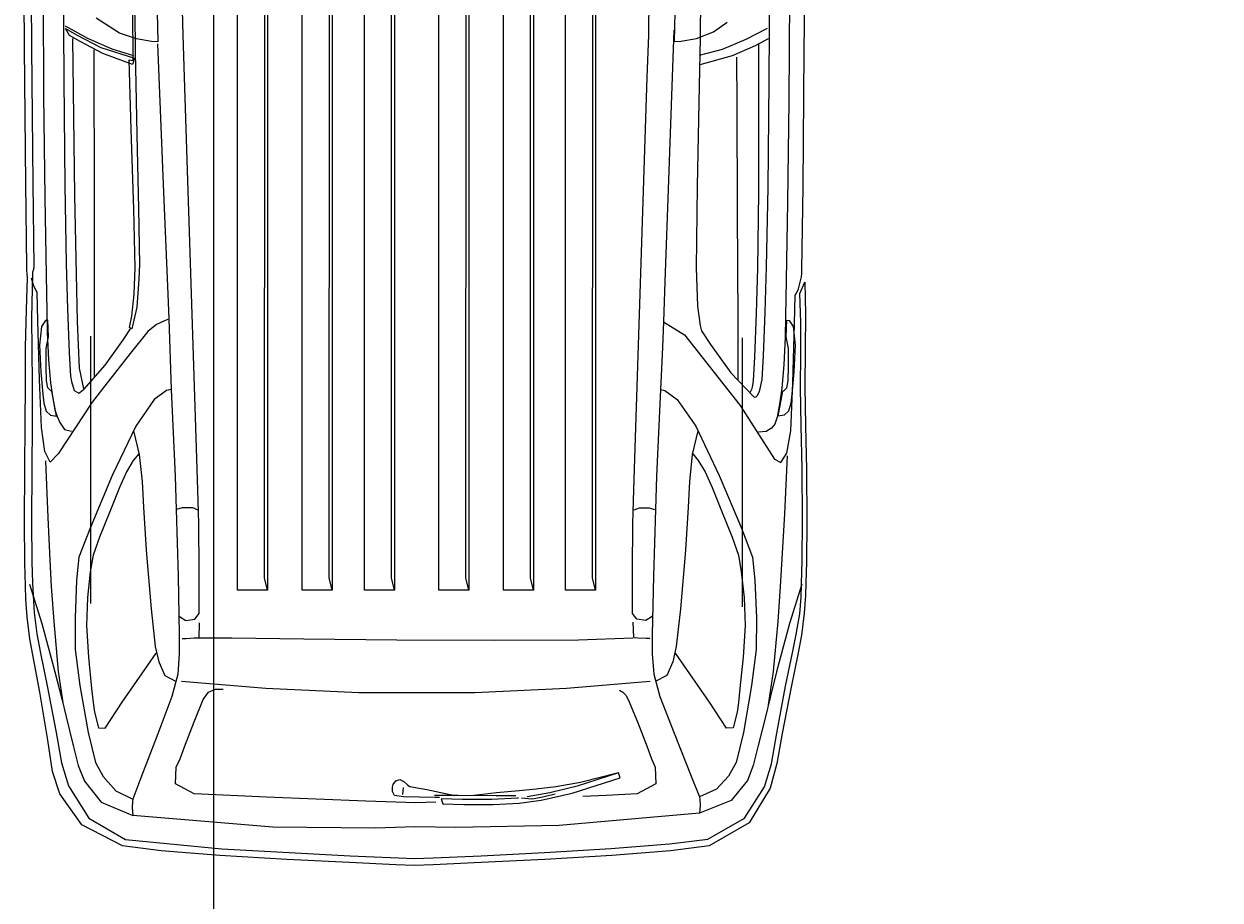
# Model space of a CAD drawing. Units: inches. Extents: x -4347 to -3836, y 955 to 1521.
# Tile 3 of 11: x -4130 to -4072, y 1023 to 1065. Entities that reach past the tile are written whole.
import ezdxf

# ---------------------------------------------------------------- set-up
doc = ezdxf.new("R2010")
doc.units = ezdxf.units.IN
doc.header["$MEASUREMENT"] = 0
doc.layers.add('A-ANNO-DIMS', color=2, linetype='Continuous', lineweight=18)
doc.layers.add('A-SITE-VEHC', color=8, linetype='Continuous', lineweight=13)
doc.styles.get("Standard").update_dxf_attribs({"font": 'arial.ttf'})
doc.dimstyles.get("Standard").update_dxf_attribs({"dimtxt": 0.18, "dimasz": 0.18, "dimexe": 0.18, "dimexo": 0.0625, "dimgap": 0.09, "dimtad": 0, "dimtih": 1, "dimtoh": 1, "dimdec": 0, "dimzin": 0, "dimdsep": 46, "dimlunit": 3, "dimtxsty": 'Standard', "dimcen": 0.09, "dimadec": 0, "dimazin": 0, "dimtfac": 1, "dimtdec": 0, "dimtofl": 0, "dimtmove": 0, "dimatfit": 3, "dimfxl": 1, "dimtolj": 1, "dimtzin": 0, "dimarcsym": 0})

# ---------------------------------------------------------------- blocks, each defined once
blk = doc.blocks.new('*D47')
at = {"layer": 'A-ANNO-DIMS', "color": 0, "lineweight": -2, "transparency": 16777216}
for p, q in [((-4120.58, 1288.726), (-4120.58, 966.959)), ((-3940.58, 1288.726), (-3940.58, 966.959)), ((-4120.4, 967.139), (-4030.97, 967.139)), ((-3940.76, 967.139), (-4030.189, 967.139))]:
    blk.add_line(p, q, dxfattribs=at)
at = {"layer": 'A-ANNO-DIMS', "color": 0, "transparency": 16777216}
for points in [[(-4120.4, 967.169), (-4120.4, 967.109), (-4120.58, 967.139)], [(-3940.76, 967.169), (-3940.76, 967.109), (-3940.58, 967.139)]]:
    blk.add_solid(points, dxfattribs=at)
at = {"layer": 'Defpoints', "color": 0, "transparency": 16777216}
for p in [(-4120.58, 1288.789), (-3940.58, 1288.789), (-3940.58, 967.139)]:
    blk.add_point(p, dxfattribs=at)
at = {"layer": 'A-ANNO-DIMS', "color": 0, "transparency": 16777216, "insert": (-4030.58, 967.139), "char_height": 0.18, "attachment_point": 5}
blk.add_mtext('\\A1;15\'-0"', dxfattribs=at)

msp = doc.modelspace()

# ---------------------------------------------------------------- linework, layer by layer
at = {"layer": 'A-SITE-VEHC'}
for p, q in [((-4119.421, 1037.674), (-4119.421, 1075.281)), ((-4117.988, 1075.281), (-4117.988, 1037.674)), ((-4117.987, 1075.281), (-4117.987, 1037.674)), ((-4116.333, 1037.674), (-4116.333, 1075.281)), ((-4114.9, 1075.281), (-4114.9, 1037.674)), ((-4114.899, 1075.281), (-4114.899, 1037.674)), ((-4113.355, 1037.674), (-4113.355, 1075.281)), ((-4111.923, 1075.281), (-4111.923, 1037.674)), ((-4111.921, 1075.281), (-4111.921, 1037.674)), ((-4109.792, 1037.674), (-4109.792, 1075.281)), ((-4108.36, 1075.281), (-4108.36, 1037.674)), ((-4108.359, 1075.281), (-4108.359, 1037.674)), ((-4106.704, 1037.674), (-4106.704, 1075.281)), ((-4105.272, 1075.281), (-4105.272, 1037.674)), ((-4105.271, 1075.281), (-4105.271, 1037.674)), ((-4103.727, 1037.674), (-4103.727, 1075.281)), ((-4102.293, 1075.281), (-4102.293, 1037.674)), ((-4118.131, 1038.272), (-4118.117, 1075.163)), ((-4115.043, 1038.272), (-4115.029, 1075.163)), ((-4112.065, 1038.272), (-4112.051, 1075.163)), ((-4108.503, 1038.272), (-4108.489, 1075.163)), ((-4105.415, 1038.272), (-4105.401, 1075.163)), ((-4102.436, 1038.272), (-4102.422, 1075.163)), ((-4127.755, 1067.874), (-4127.742, 1064.565)), ((-4123.32, 1068.019), (-4123.237, 1063.886)), ((-4098.438, 1067.866), (-4098.543, 1063.914)), ((-4097.264, 1067.866), (-4097.297, 1064.092)), ((-4094, 1067.678), (-4093.989, 1064.522)), ((-4129.614, 1063.599), (-4129.643, 1066.995)), ((-4129.312, 1066.995), (-4129.283, 1063.603)), ((-4092.31, 1063.442), (-4092.281, 1066.834)), ((-4128.73, 1066.524), (-4128.703, 1061.321)), ((-4093.024, 1066.275), (-4093.052, 1061.072)), ((-4124.346, 1065.547), (-4124.329, 1063.972)), ((-4122.033, 1064.207), (-4122.068, 1066.049)), ((-4099.752, 1064.207), (-4099.725, 1066.049)), ((-4125.067, 1064.303), (-4126.18, 1065.018)), ((-4124.412, 1063.007), (-4124.426, 1065.411)), ((-4127.742, 1064.565), (-4127.728, 1062.059)), ((-4127.664, 1064.666), (-4126.594, 1064.066)), ((-4127.466, 1064.193), (-4127.659, 1064.524)), ((-4127.659, 1064.524), (-4127.134, 1064.22)), ((-4098.545, 1064.449), (-4098.811, 1057.276)), ((-4097.463, 1064.047), (-4096.656, 1064.377)), ((-4096.656, 1064.377), (-4096.001, 1064.832)), ((-4094.088, 1064.533), (-4095.111, 1064.01)), ((-4093.989, 1064.522), (-4094.01, 1061.988)), ((-4126.958, 1063.902), (-4127.466, 1064.193)), ((-4127.314, 1064.055), (-4127.287, 1061.554)), ((-4127.134, 1064.22), (-4125.971, 1063.627)), ((-4125.876, 1063.33), (-4126.958, 1063.902)), ((-4126.594, 1064.066), (-4125.437, 1063.557)), ((-4124.25, 1064.035), (-4125.067, 1064.303)), ((-4124.329, 1063.972), (-4124.326, 1063.811)), ((-4124.326, 1063.811), (-4124.317, 1063.36)), ((-4123.54, 1063.914), (-4124.25, 1064.035)), ((-4123.237, 1063.886), (-4123.54, 1063.914)), ((-4123.249, 1063.791), (-4122.968, 1056.683)), ((-4121.96, 1062.197), (-4122.033, 1064.207)), ((-4099.825, 1062.197), (-4099.752, 1064.207)), ((-4098.543, 1063.914), (-4098.213, 1063.929)), ((-4098.213, 1063.929), (-4097.463, 1064.047)), ((-4097.297, 1064.092), (-4097.344, 1061.771)), ((-4095.111, 1064.01), (-4096.246, 1063.527)), ((-4094.642, 1063.721), (-4094.025, 1064.058)), ((-4129.553, 1057.123), (-4129.614, 1063.599)), ((-4129.283, 1063.603), (-4129.223, 1057.133)), ((-4126.294, 1063.504), (-4126.284, 1056.049)), ((-4125.971, 1063.627), (-4124.357, 1063.11)), ((-4124.453, 1062.815), (-4125.876, 1063.33)), ((-4125.437, 1063.557), (-4124.405, 1063.242)), ((-4124.317, 1063.36), (-4124.304, 1062.665)), ((-4096.246, 1063.527), (-4097.333, 1063.238)), ((-4097.297, 1062.811), (-4095.74, 1063.246)), ((-4095.74, 1063.246), (-4094.642, 1063.721)), ((-4094.504, 1063.766), (-4094.499, 1061.413)), ((-4092.371, 1056.974), (-4092.31, 1063.442)), ((-4124.508, 1059.696), (-4124.612, 1063.035)), ((-4124.612, 1063.035), (-4124.412, 1063.007)), ((-4124.357, 1063.11), (-4124.453, 1062.815)), ((-4124.304, 1062.665), (-4124.234, 1059.464)), ((-4095.552, 1063.159), (-4095.541, 1060.882)), ((-4121.831, 1058.246), (-4121.96, 1062.197)), ((-4099.954, 1058.246), (-4099.825, 1062.197)), ((-4127.728, 1062.059), (-4127.688, 1057.047)), ((-4127.287, 1061.554), (-4127.223, 1056.55)), ((-4097.344, 1061.771), (-4097.431, 1057.007)), ((-4094.01, 1061.988), (-4094.063, 1056.923)), ((-4128.703, 1061.321), (-4128.641, 1056.456)), ((-4094.499, 1061.413), (-4094.503, 1056.686)), ((-4093.052, 1061.072), (-4093.113, 1056.207)), ((-4095.541, 1060.882), (-4095.518, 1055.8)), ((-4124.39, 1055.896), (-4124.508, 1059.696)), ((-4124.234, 1059.464), (-4124.154, 1055.914)), ((-4121.675, 1053.327), (-4121.831, 1058.246)), ((-4100.11, 1053.327), (-4099.954, 1058.246)), ((-4129.501, 1053.135), (-4129.553, 1057.123)), ((-4129.223, 1057.133), (-4129.17, 1053.148)), ((-4127.688, 1057.047), (-4127.627, 1053.284)), ((-4098.811, 1057.276), (-4098.98, 1052.427)), ((-4097.431, 1057.007), (-4097.477, 1053.096)), ((-4094.063, 1056.923), (-4094.132, 1053.131)), ((-4092.423, 1052.989), (-4092.371, 1056.974)), ((-4128.641, 1056.456), (-4128.58, 1052.745)), ((-4127.223, 1056.55), (-4127.149, 1052.792)), ((-4122.968, 1056.683), (-4122.782, 1052.206)), ((-4094.503, 1056.686), (-4094.545, 1053.076)), ((-4126.284, 1056.049), (-4126.278, 1050.721)), ((-4124.323, 1053.082), (-4124.39, 1055.896)), ((-4124.154, 1055.914), (-4124.116, 1053.241)), ((-4095.518, 1055.8), (-4095.495, 1050.539)), ((-4093.113, 1056.207), (-4093.174, 1052.496)), ((-4129.496, 1052.966), (-4129.501, 1053.135)), ((-4129.488, 1052.798), (-4129.496, 1052.966)), ((-4129.19, 1053.009), (-4129.227, 1052.888)), ((-4129.17, 1053.148), (-4129.19, 1053.009)), ((-4127.627, 1053.284), (-4127.556, 1051.123)), ((-4124.365, 1051.837), (-4124.323, 1053.082)), ((-4124.116, 1053.241), (-4124.141, 1052.564)), ((-4121.518, 1048.41), (-4121.675, 1053.327)), ((-4100.267, 1048.41), (-4100.11, 1053.327)), ((-4097.477, 1053.096), (-4097.413, 1051.251)), ((-4094.545, 1053.076), (-4094.617, 1050.916)), ((-4094.132, 1053.131), (-4094.203, 1050.971)), ((-4092.434, 1052.819), (-4092.423, 1052.989)), ((-4129.527, 1051.074), (-4129.467, 1052.631)), ((-4129.467, 1052.631), (-4129.488, 1052.798)), ((-4129.165, 1052.211), (-4129.274, 1052.598)), ((-4129.231, 1052.751), (-4129.244, 1052.103)), ((-4129.227, 1052.888), (-4129.231, 1052.751)), ((-4128.58, 1052.745), (-4128.552, 1051.006)), ((-4127.149, 1052.792), (-4127.095, 1050.522)), ((-4124.141, 1052.564), (-4124.247, 1051.205)), ((-4098.98, 1052.427), (-4099.043, 1050.506)), ((-4093.174, 1052.496), (-4093.202, 1050.757)), ((-4092.581, 1052.09), (-4092.47, 1052.523)), ((-4092.519, 1051.868), (-4092.292, 1052.4)), ((-4092.47, 1052.523), (-4092.449, 1052.664)), ((-4092.449, 1052.664), (-4092.434, 1052.819)), ((-4092.292, 1052.4), (-4092.259, 1050.877)), ((-4129.244, 1052.103), (-4129.276, 1050.685)), ((-4129.061, 1051.997), (-4129.165, 1052.211)), ((-4129.015, 1051.931), (-4129.061, 1051.997)), ((-4128.983, 1050.56), (-4129.015, 1051.931)), ((-4124.477, 1050.777), (-4124.365, 1051.837)), ((-4122.782, 1052.206), (-4122.715, 1050.65)), ((-4092.775, 1050.408), (-4092.744, 1051.779)), ((-4092.744, 1051.779), (-4092.693, 1051.852)), ((-4092.693, 1051.852), (-4092.581, 1052.09)), ((-4092.48, 1050.469), (-4092.519, 1051.868)), ((-4124.247, 1051.205), (-4124.488, 1050.173)), ((-4097.413, 1051.251), (-4097.293, 1050.325)), ((-4129.562, 1049.313), (-4129.527, 1051.074)), ((-4129.276, 1050.685), (-4129.259, 1049.178)), ((-4128.552, 1051.006), (-4128.53, 1050.017)), ((-4127.556, 1051.123), (-4127.485, 1049.026)), ((-4126.278, 1050.721), (-4126.275, 1047.874)), ((-4124.598, 1050.228), (-4124.477, 1050.777)), ((-4122.759, 1050.623), (-4122.926, 1050.562)), ((-4122.715, 1050.65), (-4122.606, 1047.271)), ((-4094.617, 1050.916), (-4094.688, 1048.818)), ((-4094.203, 1050.971), (-4094.274, 1048.873)), ((-4093.202, 1050.757), (-4093.224, 1049.768)), ((-4092.259, 1050.877), (-4092.271, 1049.178)), ((-4128.904, 1047.75), (-4128.983, 1050.56)), ((-4128.805, 1050.286), (-4128.894, 1049.393)), ((-4128.605, 1050.569), (-4128.805, 1050.286)), ((-4128.493, 1050.586), (-4128.605, 1050.569)), ((-4128.473, 1049.788), (-4128.493, 1050.586)), ((-4127.095, 1050.522), (-4127.008, 1048.29)), ((-4124.53, 1050.223), (-4124.898, 1049.654)), ((-4124.488, 1050.173), (-4124.598, 1050.228)), ((-4123.712, 1050.045), (-4124.562, 1048.994)), ((-4123.304, 1050.372), (-4123.712, 1050.045)), ((-4122.926, 1050.562), (-4123.304, 1050.372)), ((-4099.043, 1050.506), (-4099.097, 1049.302)), ((-4099.043, 1050.506), (-4098.047, 1049.892)), ((-4097.293, 1050.325), (-4097.228, 1050.07)), ((-4097.228, 1050.07), (-4096.804, 1049.417)), ((-4095.495, 1050.539), (-4095.484, 1047.721)), ((-4093.173, 1049.788), (-4093.153, 1050.586)), ((-4093.153, 1050.586), (-4093.042, 1050.569)), ((-4093.042, 1050.569), (-4092.841, 1050.286)), ((-4092.854, 1047.597), (-4092.775, 1050.408)), ((-4092.841, 1050.286), (-4092.752, 1049.393)), ((-4092.483, 1048.998), (-4092.48, 1050.469)), ((-4128.574, 1049.229), (-4128.473, 1049.788)), ((-4128.53, 1050.017), (-4128.468, 1048.696)), ((-4126.46, 1049.828), (-4126.46, 1037.035)), ((-4124.898, 1049.654), (-4125.767, 1048.431)), ((-4098.047, 1049.892), (-4095.378, 1046.511)), ((-4095.275, 1049.736), (-4095.275, 1036.874)), ((-4093.224, 1049.768), (-4093.286, 1048.447)), ((-4093.072, 1049.229), (-4093.173, 1049.788)), ((-4129.574, 1047.522), (-4129.562, 1049.313)), ((-4129.259, 1049.178), (-4129.243, 1047.522)), ((-4128.894, 1049.393), (-4128.829, 1048.108)), ((-4128.578, 1048.363), (-4128.574, 1049.229)), ((-4127.485, 1049.026), (-4127.413, 1047.909)), ((-4124.562, 1048.994), (-4125.768, 1047.453)), ((-4099.097, 1049.302), (-4099.159, 1047.927)), ((-4096.804, 1049.417), (-4095.826, 1048.067)), ((-4093.068, 1048.363), (-4093.072, 1049.229)), ((-4092.752, 1049.393), (-4092.818, 1048.108)), ((-4092.492, 1047.361), (-4092.483, 1048.998)), ((-4092.271, 1049.178), (-4092.285, 1047.416)), ((-4128.562, 1047.678), (-4128.578, 1048.363)), ((-4128.468, 1048.696), (-4128.374, 1047.589)), ((-4125.767, 1048.431), (-4126.788, 1047.279)), ((-4121.389, 1044.469), (-4121.518, 1048.41)), ((-4100.395, 1044.469), (-4100.267, 1048.41)), ((-4094.688, 1048.818), (-4094.759, 1047.702)), ((-4094.274, 1048.873), (-4094.345, 1047.757)), ((-4093.286, 1048.447), (-4093.38, 1047.34)), ((-4093.084, 1047.678), (-4093.068, 1048.363)), ((-4128.829, 1048.108), (-4128.741, 1047.055)), ((-4127.413, 1047.909), (-4127.367, 1047.658)), ((-4127.008, 1048.29), (-4126.79, 1047.305)), ((-4099.159, 1047.927), (-4099.189, 1047.271)), ((-4095.826, 1048.067), (-4094.737, 1046.938)), ((-4094.345, 1047.757), (-4094.402, 1047.467)), ((-4092.818, 1048.108), (-4092.905, 1047.055)), ((-4129.583, 1045.632), (-4129.574, 1047.522)), ((-4129.243, 1047.522), (-4129.252, 1045.632)), ((-4128.802, 1045.453), (-4128.904, 1047.75)), ((-4128.498, 1047.35), (-4128.562, 1047.678)), ((-4128.378, 1047.219), (-4128.498, 1047.35)), ((-4128.314, 1047.195), (-4128.378, 1047.219)), ((-4128.374, 1047.589), (-4128.268, 1046.849)), ((-4128.079, 1045.996), (-4128.314, 1047.195)), ((-4127.367, 1047.658), (-4127.233, 1047.225)), ((-4127.233, 1047.225), (-4127.022, 1047.09)), ((-4126.946, 1047.147), (-4126.868, 1047.211)), ((-4126.868, 1047.211), (-4126.788, 1047.279)), ((-4125.768, 1047.453), (-4126.381, 1046.663)), ((-4122.819, 1047.23), (-4123.407, 1046.799)), ((-4122.606, 1047.271), (-4122.819, 1047.23)), ((-4122.606, 1047.271), (-4122.408, 1043.122)), ((-4099.189, 1047.271), (-4099.387, 1043.122)), ((-4099.189, 1047.271), (-4098.975, 1047.23)), ((-4098.975, 1047.23), (-4098.388, 1046.799)), ((-4094.831, 1047.268), (-4094.918, 1047.112)), ((-4094.795, 1047.47), (-4094.831, 1047.268)), ((-4094.759, 1047.702), (-4094.795, 1047.47)), ((-4094.402, 1047.467), (-4094.477, 1047.159)), ((-4093.567, 1045.996), (-4093.333, 1047.195)), ((-4093.38, 1047.34), (-4093.491, 1046.567)), ((-4093.333, 1047.195), (-4093.268, 1047.219)), ((-4093.268, 1047.219), (-4093.149, 1047.35)), ((-4093.149, 1047.35), (-4093.084, 1047.678)), ((-4092.957, 1045.301), (-4092.854, 1047.597)), ((-4092.467, 1045.54), (-4092.492, 1047.361)), ((-4092.285, 1047.416), (-4092.259, 1045.553)), ((-4128.741, 1047.055), (-4128.698, 1046.619)), ((-4128.698, 1046.619), (-4128.586, 1046.235)), ((-4128.268, 1046.849), (-4128.161, 1046.3)), ((-4126.381, 1046.663), (-4128.003, 1044.19)), ((-4127.022, 1047.09), (-4126.946, 1047.147)), ((-4123.407, 1046.799), (-4124.288, 1045.517)), ((-4098.388, 1046.799), (-4097.506, 1045.517)), ((-4094.737, 1046.938), (-4094.68, 1046.911)), ((-4094.68, 1046.911), (-4094.629, 1046.915)), ((-4094.629, 1046.915), (-4094.584, 1046.945)), ((-4094.477, 1047.159), (-4094.584, 1046.945)), ((-4092.949, 1046.619), (-4093.06, 1046.235)), ((-4092.905, 1047.055), (-4092.949, 1046.619)), ((-4128.586, 1046.235), (-4128.371, 1046.05)), ((-4128.371, 1046.05), (-4128.079, 1045.996)), ((-4128.161, 1046.3), (-4128.054, 1045.987)), ((-4095.378, 1046.511), (-4093.732, 1043.942)), ((-4093.491, 1046.567), (-4093.607, 1045.955)), ((-4093.275, 1046.05), (-4093.567, 1045.996)), ((-4093.06, 1046.235), (-4093.275, 1046.05)), ((-4129.6, 1043.456), (-4129.583, 1045.632)), ((-4129.252, 1045.632), (-4129.27, 1043.456)), ((-4128.054, 1045.987), (-4127.921, 1045.694)), ((-4127.921, 1045.694), (-4127.707, 1045.362)), ((-4124.288, 1045.517), (-4125.416, 1043.152)), ((-4097.506, 1045.517), (-4096.379, 1043.152)), ((-4093.719, 1045.61), (-4093.872, 1045.419)), ((-4093.607, 1045.955), (-4093.719, 1045.61)), ((-4092.42, 1043.492), (-4092.467, 1045.54)), ((-4092.259, 1045.553), (-4092.211, 1043.429)), ((-4128.648, 1044.303), (-4128.802, 1045.453)), ((-4127.707, 1045.362), (-4127.369, 1045.279)), ((-4124.396, 1045.302), (-4124.124, 1044.156)), ((-4097.399, 1045.302), (-4097.671, 1044.156)), ((-4094.128, 1045.264), (-4094.504, 1045.238)), ((-4093.872, 1045.419), (-4094.128, 1045.264)), ((-4093.147, 1044.232), (-4092.957, 1045.301)), ((-4121.317, 1042.474), (-4121.389, 1044.469)), ((-4100.468, 1042.474), (-4100.395, 1044.469)), ((-4128.389, 1043.798), (-4128.648, 1044.303)), ((-4128.61, 1043.859), (-4128.499, 1041.149)), ((-4128.003, 1044.19), (-4128.389, 1043.798)), ((-4124.41, 1043.87), (-4124.739, 1043.333)), ((-4124.145, 1044.192), (-4124.41, 1043.87)), ((-4124.124, 1044.156), (-4123.987, 1042.867)), ((-4097.671, 1044.156), (-4097.807, 1042.867)), ((-4097.649, 1044.192), (-4097.384, 1043.87)), ((-4097.384, 1043.87), (-4097.055, 1043.333)), ((-4093.732, 1043.942), (-4093.439, 1043.787)), ((-4093.439, 1043.787), (-4093.147, 1044.232)), ((-4093.126, 1044.107), (-4093.252, 1041.332)), ((-4129.61, 1040.97), (-4129.6, 1043.456)), ((-4129.27, 1043.456), (-4129.279, 1040.97)), ((-4124.739, 1043.333), (-4125.076, 1042.581)), ((-4097.055, 1043.333), (-4096.718, 1042.581)), ((-4092.395, 1041.074), (-4092.42, 1043.492)), ((-4092.211, 1043.429), (-4092.185, 1040.97)), ((-4125.416, 1043.152), (-4126.479, 1040.637)), ((-4123.987, 1042.867), (-4123.93, 1041.65)), ((-4122.408, 1043.122), (-4122.266, 1038.352)), ((-4099.387, 1043.122), (-4099.528, 1038.352)), ((-4097.807, 1042.867), (-4097.864, 1041.65)), ((-4096.379, 1043.152), (-4095.315, 1040.637)), ((-4125.076, 1042.581), (-4125.52, 1041.467)), ((-4121.276, 1040.866), (-4121.317, 1042.474)), ((-4100.508, 1040.866), (-4100.468, 1042.474)), ((-4096.718, 1042.581), (-4096.274, 1041.467)), ((-4125.52, 1041.467), (-4126.028, 1040.21)), ((-4123.93, 1041.65), (-4123.798, 1039.589)), ((-4122.324, 1041.543), (-4122.063, 1041.626)), ((-4122.063, 1041.626), (-4121.58, 1041.623)), ((-4121.58, 1041.623), (-4121.324, 1041.522)), ((-4100.204, 1041.595), (-4100.46, 1041.495)), ((-4099.722, 1041.599), (-4100.204, 1041.595)), ((-4099.461, 1041.515), (-4099.722, 1041.599)), ((-4097.864, 1041.65), (-4097.997, 1039.589)), ((-4096.274, 1041.467), (-4095.766, 1040.21)), ((-4129.594, 1038.961), (-4129.61, 1040.97)), ((-4129.279, 1040.97), (-4129.26, 1039.008)), ((-4128.499, 1041.149), (-4128.398, 1039.109)), ((-4093.252, 1041.332), (-4093.381, 1039.173)), ((-4092.413, 1039.063), (-4092.395, 1041.074)), ((-4092.185, 1040.97), (-4092.203, 1039.008)), ((-4126.479, 1040.637), (-4127.009, 1039.251)), ((-4121.258, 1038.624), (-4121.276, 1040.866)), ((-4100.527, 1038.624), (-4100.508, 1040.866)), ((-4095.315, 1040.637), (-4094.785, 1039.251)), ((-4126.028, 1040.21), (-4126.329, 1039.358)), ((-4095.766, 1040.21), (-4095.465, 1039.358)), ((-4127.009, 1039.251), (-4127.12, 1038.157)), ((-4126.329, 1039.358), (-4126.469, 1038.557)), ((-4123.798, 1039.589), (-4123.562, 1036.788)), ((-4097.997, 1039.589), (-4098.233, 1036.788)), ((-4095.465, 1039.358), (-4095.326, 1038.557)), ((-4094.785, 1039.251), (-4094.675, 1038.157)), ((-4093.381, 1039.173), (-4093.46, 1037.855)), ((-4129.564, 1037.89), (-4129.594, 1038.961)), ((-4129.26, 1039.008), (-4129.226, 1038.026)), ((-4128.398, 1039.109), (-4128.334, 1037.855)), ((-4121.257, 1036.556), (-4121.258, 1038.624)), ((-4100.528, 1036.556), (-4100.527, 1038.624)), ((-4092.446, 1037.989), (-4092.413, 1039.063)), ((-4092.203, 1039.008), (-4092.238, 1038.026)), ((-4127.12, 1038.157), (-4127.198, 1036.347)), ((-4126.469, 1038.557), (-4126.608, 1037.319)), ((-4122.266, 1038.352), (-4122.212, 1035.563)), ((-4117.988, 1037.674), (-4118.131, 1038.272)), ((-4114.9, 1037.674), (-4115.043, 1038.272)), ((-4111.923, 1037.674), (-4112.065, 1038.272)), ((-4108.36, 1037.674), (-4108.503, 1038.272)), ((-4105.272, 1037.674), (-4105.415, 1038.272)), ((-4102.293, 1037.674), (-4102.436, 1038.272)), ((-4099.528, 1038.352), (-4099.583, 1035.563)), ((-4095.326, 1038.557), (-4095.187, 1037.319)), ((-4094.675, 1038.157), (-4094.597, 1036.347)), ((-4129.548, 1037.242), (-4129.564, 1037.89)), ((-4129.373, 1037.962), (-4128.783, 1036.08)), ((-4129.226, 1038.026), (-4129.207, 1037.425)), ((-4128.334, 1037.855), (-4128.218, 1036.173)), ((-4117.987, 1037.674), (-4119.421, 1037.674)), ((-4114.899, 1037.674), (-4116.333, 1037.674)), ((-4111.921, 1037.674), (-4113.355, 1037.674)), ((-4108.359, 1037.674), (-4109.792, 1037.674)), ((-4105.271, 1037.674), (-4106.704, 1037.674)), ((-4102.293, 1037.674), (-4103.727, 1037.674)), ((-4093.46, 1037.855), (-4093.577, 1036.173)), ((-4092.422, 1037.962), (-4093.012, 1036.08)), ((-4092.464, 1037.338), (-4092.446, 1037.989)), ((-4092.238, 1038.026), (-4092.256, 1037.425)), ((-4129.494, 1036.4), (-4129.548, 1037.242)), ((-4129.207, 1037.425), (-4129.155, 1036.612)), ((-4126.608, 1037.319), (-4126.652, 1035.993)), ((-4095.187, 1037.319), (-4095.143, 1035.993)), ((-4092.532, 1036.549), (-4092.464, 1037.338)), ((-4092.256, 1037.425), (-4092.31, 1036.583)), ((-4129.36, 1035.345), (-4129.494, 1036.4)), ((-4129.155, 1036.612), (-4129.024, 1035.582)), ((-4127.198, 1036.347), (-4127.189, 1034.847)), ((-4123.562, 1036.788), (-4123.357, 1034.99)), ((-4122.198, 1036.419), (-4121.89, 1036.233)), ((-4121.469, 1036.292), (-4121.257, 1036.556)), ((-4100.316, 1036.292), (-4100.528, 1036.556)), ((-4099.587, 1036.419), (-4099.895, 1036.233)), ((-4098.233, 1036.788), (-4098.437, 1034.99)), ((-4094.597, 1036.347), (-4094.606, 1034.847)), ((-4092.692, 1035.565), (-4092.532, 1036.549)), ((-4092.31, 1036.583), (-4092.444, 1035.528)), ((-4128.783, 1036.08), (-4128.161, 1033.769)), ((-4128.218, 1036.173), (-4127.998, 1033.783)), ((-4126.652, 1035.993), (-4126.552, 1034.48)), ((-4121.89, 1036.233), (-4121.469, 1036.292)), ((-4121.257, 1036.118), (-4121.281, 1035.384)), ((-4100.506, 1036.149), (-4100.483, 1035.415)), ((-4099.895, 1036.233), (-4100.316, 1036.292)), ((-4095.143, 1035.993), (-4095.243, 1034.48)), ((-4093.577, 1036.173), (-4093.797, 1033.783)), ((-4093.012, 1036.08), (-4093.634, 1033.769)), ((-4129.185, 1034.411), (-4129.36, 1035.345)), ((-4129.024, 1035.582), (-4128.854, 1034.67)), ((-4122.212, 1035.563), (-4122.209, 1034.633)), ((-4121.88, 1035.357), (-4122.068, 1035.348)), ((-4121.493, 1035.375), (-4121.88, 1035.357)), ((-4121.281, 1035.384), (-4121.493, 1035.375)), ((-4119.691, 1035.377), (-4121.281, 1035.384)), ((-4116.259, 1035.336), (-4119.691, 1035.377)), ((-4111.804, 1035.29), (-4116.259, 1035.336)), ((-4107.147, 1035.265), (-4111.804, 1035.29)), ((-4103.11, 1035.287), (-4107.147, 1035.265)), ((-4100.514, 1035.384), (-4103.11, 1035.287)), ((-4100.483, 1035.415), (-4100.27, 1035.405)), ((-4100.27, 1035.405), (-4099.883, 1035.388)), ((-4099.883, 1035.388), (-4099.695, 1035.379)), ((-4099.583, 1035.563), (-4099.585, 1034.633)), ((-4092.878, 1034.678), (-4092.692, 1035.565)), ((-4092.444, 1035.528), (-4092.619, 1034.594)), ((-4128.854, 1034.67), (-4128.529, 1033.103)), ((-4127.189, 1034.847), (-4126.962, 1033.127)), ((-4123.865, 1033.891), (-4123.322, 1034.668)), ((-4123.357, 1034.99), (-4123.193, 1034.244)), ((-4122.209, 1034.633), (-4122.286, 1033.664)), ((-4099.585, 1034.633), (-4099.509, 1033.664)), ((-4098.437, 1034.99), (-4098.601, 1034.244)), ((-4097.929, 1033.891), (-4098.473, 1034.668)), ((-4094.606, 1034.847), (-4094.833, 1033.127)), ((-4093.202, 1033.094), (-4092.878, 1034.678)), ((-4092.619, 1034.594), (-4092.941, 1033.037)), ((-4128.885, 1032.805), (-4129.185, 1034.411)), ((-4126.552, 1034.48), (-4126.405, 1032.982)), ((-4123.193, 1034.244), (-4122.901, 1033.6)), ((-4098.601, 1034.244), (-4098.893, 1033.6)), ((-4095.243, 1034.48), (-4095.39, 1032.982)), ((-4128.161, 1033.769), (-4127.833, 1032.484)), ((-4127.998, 1033.783), (-4127.762, 1032.197)), ((-4124.95, 1032.318), (-4123.865, 1033.891)), ((-4122.901, 1033.6), (-4122.355, 1033.307)), ((-4122.286, 1033.664), (-4122.57, 1032.591)), ((-4099.509, 1033.664), (-4099.225, 1032.591)), ((-4098.893, 1033.6), (-4099.44, 1033.307)), ((-4096.844, 1032.318), (-4097.929, 1033.891)), ((-4093.797, 1033.783), (-4094.033, 1032.197)), ((-4093.634, 1033.769), (-4093.961, 1032.484)), ((-4128.529, 1033.103), (-4128.101, 1030.873)), ((-4126.962, 1033.127), (-4126.568, 1030.874)), ((-4126.405, 1032.982), (-4126.329, 1032.305)), ((-4118.074, 1032.969), (-4122.104, 1033.307)), ((-4120.808, 1032.806), (-4120.481, 1032.947)), ((-4120.481, 1032.947), (-4120.119, 1032.951)), ((-4113.615, 1032.774), (-4118.074, 1032.969)), ((-4103.683, 1032.969), (-4108.074, 1032.774)), ((-4099.69, 1033.307), (-4103.683, 1032.969)), ((-4101.144, 1032.899), (-4100.987, 1032.807)), ((-4095.39, 1032.982), (-4095.465, 1032.305)), ((-4094.833, 1033.127), (-4095.227, 1030.874)), ((-4093.631, 1030.834), (-4093.202, 1033.094)), ((-4092.941, 1033.037), (-4093.367, 1030.822)), ((-4128.502, 1030.5), (-4128.885, 1032.805)), ((-4127.833, 1032.484), (-4127.621, 1031.626)), ((-4126.329, 1032.305), (-4126.268, 1031.838)), ((-4125.756, 1031.087), (-4124.95, 1032.318)), ((-4122.57, 1032.591), (-4123.243, 1030.811)), ((-4121.497, 1031.38), (-4121.066, 1032.448)), ((-4121.066, 1032.448), (-4120.808, 1032.806)), ((-4110.826, 1032.77), (-4113.615, 1032.774)), ((-4108.074, 1032.774), (-4110.826, 1032.77)), ((-4100.987, 1032.807), (-4100.847, 1032.66)), ((-4100.847, 1032.66), (-4100.729, 1032.448)), ((-4100.729, 1032.448), (-4100.298, 1031.38)), ((-4099.225, 1032.591), (-4098.539, 1030.84)), ((-4096.038, 1031.087), (-4096.844, 1032.318)), ((-4095.465, 1032.305), (-4095.526, 1031.838)), ((-4093.961, 1032.484), (-4094.174, 1031.626)), ((-4126.268, 1031.838), (-4126.08, 1031.101)), ((-4095.526, 1031.838), (-4095.715, 1031.101)), ((-4127.621, 1031.626), (-4127.281, 1030.251)), ((-4121.96, 1030.186), (-4121.497, 1031.38)), ((-4100.298, 1031.38), (-4099.835, 1030.186)), ((-4094.174, 1031.626), (-4094.513, 1030.251)), ((-4128.101, 1030.873), (-4127.848, 1029.425)), ((-4126.568, 1030.874), (-4126.222, 1029.44)), ((-4126.08, 1031.101), (-4125.756, 1031.087)), ((-4123.243, 1030.811), (-4124.044, 1028.706)), ((-4098.539, 1030.84), (-4097.716, 1028.788)), ((-4095.715, 1031.101), (-4096.038, 1031.087)), ((-4095.227, 1030.874), (-4095.573, 1029.44)), ((-4093.884, 1029.37), (-4093.631, 1030.834)), ((-4093.367, 1030.822), (-4093.618, 1029.384)), ((-4128.273, 1029.014), (-4128.502, 1030.5)), ((-4127.281, 1030.251), (-4127.045, 1029.297)), ((-4122.176, 1029.619), (-4121.96, 1030.186)), ((-4099.835, 1030.186), (-4099.619, 1029.619)), ((-4094.513, 1030.251), (-4094.749, 1029.297)), ((-4122.358, 1029.207), (-4122.176, 1029.619)), ((-4099.619, 1029.619), (-4099.437, 1029.207)), ((-4127.918, 1027.942), (-4128.273, 1029.014)), ((-4127.848, 1029.425), (-4127.511, 1028.319)), ((-4127.045, 1029.297), (-4126.752, 1028.541)), ((-4126.222, 1029.44), (-4125.853, 1028.764)), ((-4122.388, 1028.421), (-4122.358, 1029.207)), ((-4101.193, 1028.943), (-4103.169, 1028.307)), ((-4101.193, 1028.943), (-4103.011, 1028.487)), ((-4101.121, 1028.705), (-4101.193, 1028.943)), ((-4099.437, 1029.207), (-4099.406, 1028.421)), ((-4095.573, 1029.44), (-4095.929, 1028.792)), ((-4094.749, 1029.297), (-4095.031, 1028.57)), ((-4094.215, 1028.282), (-4093.884, 1029.37)), ((-4093.618, 1029.384), (-4093.948, 1028.216)), ((-4127.511, 1028.319), (-4126.539, 1026.779)), ((-4126.752, 1028.541), (-4125.949, 1027.54)), ((-4125.853, 1028.764), (-4125.254, 1028.08)), ((-4124.044, 1028.706), (-4124.432, 1027.69)), ((-4121.496, 1027.937), (-4122.388, 1028.421)), ((-4112.012, 1028.254), (-4111.975, 1028.392)), ((-4111.975, 1028.392), (-4111.847, 1028.554)), ((-4111.847, 1028.554), (-4111.667, 1028.626)), ((-4111.667, 1028.626), (-4111.47, 1028.535)), ((-4111.47, 1028.535), (-4111.292, 1028.374)), ((-4111.292, 1028.374), (-4111.162, 1028.275)), ((-4103.169, 1028.307), (-4104.483, 1027.992)), ((-4103.011, 1028.487), (-4104.19, 1028.274)), ((-4103.418, 1027.974), (-4101.121, 1028.705)), ((-4099.406, 1028.421), (-4100.299, 1027.937)), ((-4097.716, 1028.788), (-4097.317, 1027.801)), ((-4095.929, 1028.792), (-4096.506, 1028.162)), ((-4095.031, 1028.57), (-4095.811, 1027.621)), ((-4126.868, 1026.461), (-4127.918, 1027.942)), ((-4125.254, 1028.08), (-4124.432, 1027.69)), ((-4118.032, 1027.777), (-4121.496, 1027.937)), ((-4113.287, 1027.594), (-4118.032, 1027.777)), ((-4112.006, 1028.045), (-4112.012, 1028.254)), ((-4111.913, 1027.861), (-4112.006, 1028.045)), ((-4111.484, 1027.796), (-4111.913, 1027.861)), ((-4111.51, 1027.911), (-4111.487, 1028.235)), ((-4109.981, 1027.759), (-4111.484, 1027.796)), ((-4111.003, 1028.248), (-4111.162, 1028.275)), ((-4110.369, 1028.126), (-4111.003, 1028.248)), ((-4109.022, 1027.852), (-4110.369, 1028.126)), ((-4108.874, 1027.854), (-4109.995, 1027.86)), ((-4109.768, 1027.757), (-4109.981, 1027.759)), ((-4107.056, 1027.85), (-4108.874, 1027.854)), ((-4107.031, 1027.981), (-4108.119, 1027.855)), ((-4106.029, 1027.735), (-4107.266, 1027.666)), ((-4106.104, 1027.848), (-4107.056, 1027.85)), ((-4105.948, 1028.08), (-4107.031, 1027.981)), ((-4106.015, 1027.736), (-4106.029, 1027.735)), ((-4106.001, 1027.738), (-4106.015, 1027.736)), ((-4105.987, 1027.74), (-4106.001, 1027.738)), ((-4105.142, 1028.158), (-4105.948, 1028.08)), ((-4105.323, 1027.689), (-4105.846, 1027.729)), ((-4104.483, 1027.992), (-4105.568, 1027.803)), ((-4104.754, 1027.803), (-4105.16, 1027.72)), ((-4104.19, 1028.274), (-4105.142, 1028.158)), ((-4104.9, 1027.64), (-4103.418, 1027.974)), ((-4104.228, 1027.926), (-4104.754, 1027.803)), ((-4101.795, 1027.861), (-4102.902, 1027.813)), ((-4100.903, 1027.903), (-4101.795, 1027.861)), ((-4100.299, 1027.937), (-4100.903, 1027.903)), ((-4096.506, 1028.162), (-4097.317, 1027.801)), ((-4097.317, 1027.801), (-4097.301, 1027.676)), ((-4095.175, 1026.774), (-4094.215, 1028.282)), ((-4093.948, 1028.216), (-4094.952, 1026.557)), ((-4125.949, 1027.54), (-4124.432, 1026.902)), ((-4124.448, 1027.566), (-4124.463, 1027.266)), ((-4124.463, 1027.266), (-4124.432, 1026.902)), ((-4124.432, 1027.69), (-4124.448, 1027.566)), ((-4110.897, 1027.507), (-4113.287, 1027.594)), ((-4109.944, 1027.541), (-4110.897, 1027.507)), ((-4108.663, 1027.666), (-4109.681, 1027.697)), ((-4109.681, 1027.697), (-4109.608, 1027.459)), ((-4109.608, 1027.459), (-4108.591, 1027.428)), ((-4107.266, 1027.666), (-4108.663, 1027.666)), ((-4108.591, 1027.428), (-4107.193, 1027.428)), ((-4107.193, 1027.428), (-4105.957, 1027.497)), ((-4105.957, 1027.497), (-4104.9, 1027.64)), ((-4105.16, 1027.72), (-4105.323, 1027.689)), ((-4095.811, 1027.621), (-4097.317, 1027.013)), ((-4097.285, 1027.376), (-4097.317, 1027.013)), ((-4097.301, 1027.676), (-4097.285, 1027.376)), ((-4126.539, 1026.779), (-4124.778, 1025.758)), ((-4117.733, 1026.348), (-4124.432, 1026.902)), ((-4097.317, 1027.013), (-4104.045, 1026.43)), ((-4096.93, 1025.771), (-4095.175, 1026.774)), ((-4124.929, 1025.447), (-4126.868, 1026.461)), ((-4112.833, 1026.295), (-4117.733, 1026.348)), ((-4110.933, 1026.361), (-4112.833, 1026.295)), ((-4109.002, 1026.323), (-4110.933, 1026.361)), ((-4104.045, 1026.43), (-4109.002, 1026.323)), ((-4094.952, 1026.557), (-4096.865, 1025.447)), ((-4123.084, 1025.215), (-4124.929, 1025.447)), ((-4124.778, 1025.758), (-4120.171, 1025.316)), ((-4101.561, 1025.325), (-4098.764, 1025.542)), ((-4098.764, 1025.542), (-4096.93, 1025.771)), ((-4096.865, 1025.447), (-4098.71, 1025.215)), ((-4120.27, 1024.997), (-4123.084, 1025.215)), ((-4117.069, 1024.804), (-4120.27, 1024.997)), ((-4120.171, 1025.316), (-4114.035, 1024.978)), ((-4114.035, 1024.978), (-4110.962, 1024.844)), ((-4110.962, 1024.844), (-4110.059, 1024.88)), ((-4110.059, 1024.88), (-4107.773, 1024.981)), ((-4107.773, 1024.981), (-4104.743, 1025.134)), ((-4104.743, 1025.134), (-4101.561, 1025.325)), ((-4101.524, 1024.997), (-4104.725, 1024.804)), ((-4098.71, 1025.215), (-4101.524, 1024.997)), ((-4114.071, 1024.651), (-4117.069, 1024.804)), ((-4111.846, 1024.55), (-4114.071, 1024.651)), ((-4110.976, 1024.513), (-4111.846, 1024.55)), ((-4110.065, 1024.55), (-4110.976, 1024.513)), ((-4107.765, 1024.651), (-4110.065, 1024.55)), ((-4104.725, 1024.804), (-4107.765, 1024.651))]:
    msp.add_line(p, q, dxfattribs=at)

# ---------------------------------------------------------------- dimensions: what is measured, and where the dimension line sits
at = {"layer": 'A-ANNO-DIMS'}
dim = msp.add_linear_dim(base=(-3940.58, 967.139), p1=(-4120.58, 1288.789), p2=(-3940.58, 1288.789), dimstyle='Standard', override={"dimdec": 1, "dimlfac": 1, "dimrnd": 0, "dimzin": 1, "dimdsep": 46, "dimlunit": 4, "dimfrac": 2}, dxfattribs=at)
dim.commit()
dim.dimension.update_dxf_attribs({"geometry": '*D47', "text_midpoint": (-4030.58, 967.139)})

doc.saveas('drawing.dxf')
